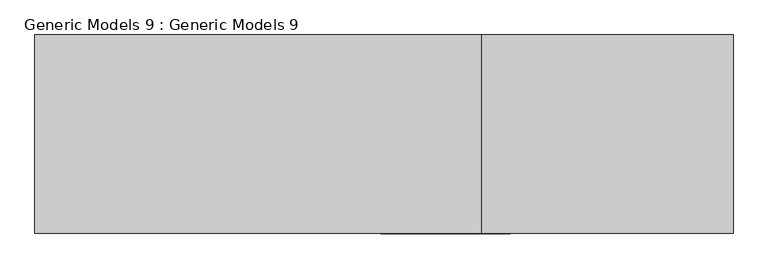
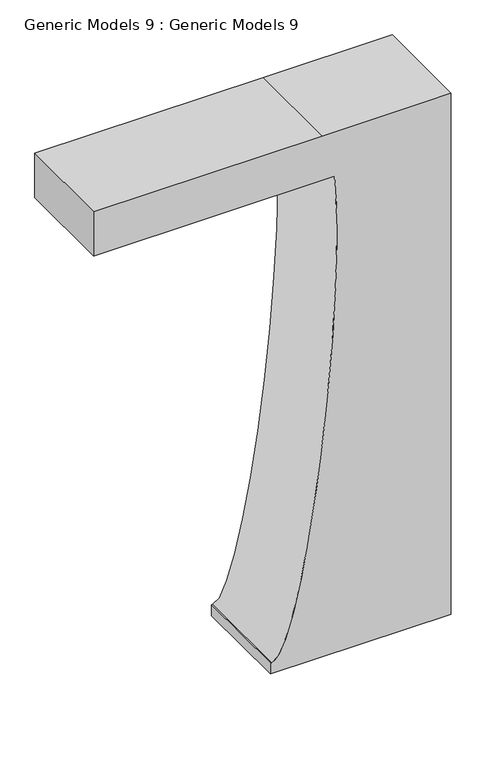
"""IFC4 building model written with IfcOpenShell, lengths in millimetres: proxy geometry, Generic Models 9 : Generic Models 9."""

from ifc_helpers import new_model, si_unit, point, frame, origin, place, context, project, spatial, ellipse_curve, trimmed, source, transform, mapped, element, save
from ifc_brep_helpers import plane_surface, extruded_surface, advanced_brep


def generic_models_9_generic_models_9_71cd0b1b(model_context):
    return source(origin(), model_context, "Body", "AdvancedBrep", [
        advanced_brep(
        [(-10072.6353949, -1359.4088252, 0.0), (-12767.6856484, -1359.4088252, 0.0), (-12767.6856484, -1359.4088252, 173.9941328), (-12752.3257402, -1359.4088252, 173.9941328), (-11811.6414408, -1359.4088252, 7525.2735957), (-15409.4848607, -1359.4088252, 7525.2735957), (-15409.4848607, -1359.4088252, 8225.5499862), (-11999.3356484, -1359.4088252, 8225.5499862), (-10072.6353949, -1359.4088252, 8225.5499862), (-10072.6353949, -2877.1333439, 0.0), (-10072.6353949, -2877.1333439, 8225.5499862), (-11999.3356484, -2877.1333439, 8225.5499862), (-15409.4848607, -2877.1333439, 8225.5499862), (-15409.4848607, -2877.1333439, 7525.2735957), (-11811.6414408, -2877.1333439, 7525.2735957), (-12752.3257402, -2877.1333439, 173.9941328), (-12767.6856484, -2877.1333439, 173.9941328), (-12767.6856484, -2877.1333439, 0.0)],
        [
            (0, 1),
            (1, 2),
            (2, 3),
            (3, 4, ellipse_curve(frame((-12370.1794548, -1359.4088252, 4125.5970664), z_axis=(0.0, -1.0, 0.0), x_axis=(0.09625758940780418, 0.0, 0.9953564569948791)), 3970.0379756, 457.2)),
            (4, 5),
            (5, 6),
            (6, 7),
            (7, 8),
            (8, 0),
            (9, 10),
            (10, 11),
            (11, 12),
            (12, 13),
            (13, 14),
            (14, 15, ellipse_curve(frame((-12370.1794548, -2877.1333439, 4125.5970664), z_axis=(0.0, 1.0, 0.0), x_axis=(0.09625758940780418, 0.0, 0.9953564569948791)), 3970.0379756, 457.2)),
            (15, 16),
            (16, 17),
            (17, 9),
            (0, 9),
            (17, 1),
            (16, 2),
            (15, 3),
            (14, 4),
            (13, 5),
            (12, 6),
            (11, 7),
            (10, 8),
        ],
        [
            plane_surface(frame((-11732.6356484, -1359.4088252, 0.0), z_axis=(0.0, 1.0, 0.0), x_axis=(-1.0, 0.0, 0.0))),
            plane_surface(frame((-11732.6356484, -2877.1333439, 0.0), z_axis=(0.0, -1.0, 0.0), x_axis=(1.0, 0.0, 0.0))),
            plane_surface(frame((-10072.6353949, -1359.4088252, 0.0), z_axis=(0.0, 0.0, -1.0), x_axis=(0.0, -1.0, 0.0))),
            plane_surface(frame((-12767.6856484, -1359.4088252, 0.0), z_axis=(-1.0, 0.0, 0.0), x_axis=(0.0, -1.0, 0.0))),
            plane_surface(frame((-12767.6856484, -1359.4088252, 173.9941328), z_axis=(0.0, 0.0, 1.0), x_axis=(0.0, -1.0, 0.0))),
            extruded_surface(trimmed(ellipse_curve(frame((-12370.1794548, -4394.8578626, 4125.5970664), z_axis=(0.0, -1.0, 0.0), x_axis=(0.09625758940780418, 0.0, 0.9953564569948791)), 3970.0379756, 457.2), [point((-12752.3257402, -4394.8578626, 173.9941328))], [point((-11811.6414408, -4394.8578626, 7525.2735957))], True, "CARTESIAN"), (0.0, 1517.7245186999999, 0.0), 1517.7245186999999),
            plane_surface(frame((-11811.6414408, -1359.4088252, 7525.2735957), z_axis=(0.0, 0.0, -1.0), x_axis=(0.0, -1.0, 0.0))),
            plane_surface(frame((-15409.4848607, -1359.4088252, 7525.2735957), z_axis=(-1.0, 0.0, 0.0), x_axis=(0.0, -1.0, 0.0))),
            plane_surface(frame((-15409.4848607, -1359.4088252, 8225.5499862), z_axis=(0.0, 0.0, 1.0), x_axis=(0.0, -1.0, 0.0))),
            plane_surface(frame((-11999.3356484, -1359.4088252, 8225.5499862), z_axis=(0.0, 0.0, 1.0), x_axis=(0.0, -1.0, 0.0))),
            plane_surface(frame((-10072.6353949, -1359.4088252, 8225.5499862), z_axis=(1.0, 0.0, 0.0), x_axis=(0.0, -1.0, 0.0))),
        ],
        [
            (0, [[1, 2, 3, 4, 5, 6, 7, 8, 9]]),
            (1, [[10, 11, 12, 13, 14, 15, 16, 17, 18]]),
            (2, [[-1, 19, -18, 20]]),
            (3, [[-2, -20, -17, 21]]),
            (4, [[-3, -21, -16, 22]]),
            (5, [[-4, -22, -15, 23]]),
            (6, [[-5, -23, -14, 24]]),
            (7, [[-6, -24, -13, 25]]),
            (8, [[-7, -25, -12, 26]]),
            (9, [[-8, -26, -11, 27]]),
            (10, [[-9, -27, -10, -19]]),
        ],
    ),
    ])


if __name__ == "__main__":
    model = new_model("IFC4")
    model_context = context("Model", 3, world=origin())
    ifc_project = project(units=[si_unit("LENGTHUNIT", "METRE", prefix="MILLI")], contexts=[model_context])
    site = spatial("IfcSite", under=ifc_project)
    building = spatial("IfcBuilding", under=site)
    placement = place(None, origin())
    generic_models_9_generic_models_9_shape = generic_models_9_generic_models_9_71cd0b1b(model_context)
    element("IfcBuildingElementProxy", 1, Name="Generic Models 9 : Generic Models 9", ObjectType="Generic Models 9 : Generic Models 9", at=placement, inside=building, context=model_context, shape_type="MappedRepresentation", body=[
        mapped(generic_models_9_generic_models_9_shape, transform((0.0, 0.0, 0.0), x_axis=(1.0, 0.0, 0.0), y_axis=(0.0, 1.0, 0.0), z_axis=(0.0, 0.0, 1.0))),
    ])
    save(model, "model.ifc")
